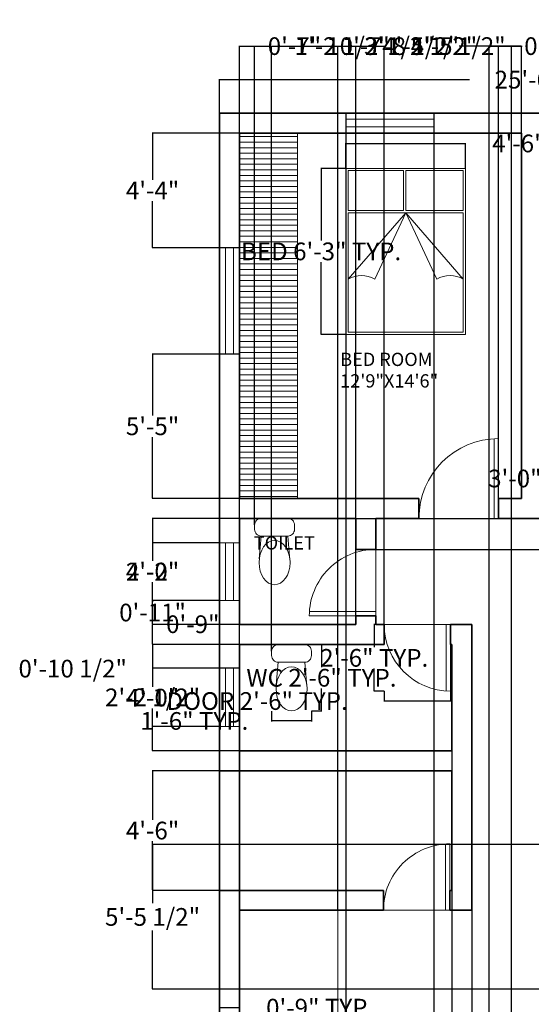
# Model space of a CAD drawing. Units: inches. Extents: x -69 to 405, y -4 to 680.
# Tile 2 of 3: x -69 to 162, y 236 to 680. Entities that reach past the tile are written whole.
import ezdxf

# ---------------------------------------------------------------- set-up
doc = ezdxf.new("R2010")
doc.units = ezdxf.units.IN
doc.header["$MEASUREMENT"] = 0
for name, color, linetype, lineweight in [('A-ANNO-DIMS', 4, 'Continuous', 18), ('A-AREA-IDEN', 4, 'Continuous', 18), ('A-FLOR-CASE', 7, 'Continuous', 18), ('A-FLOR-FIXT', 8, 'Continuous', 18), ('A-WALL', 7, 'Continuous', 35), ('Furniture', 7, 'Continuous', 15)]:
    doc.layers.add(name, color=color, linetype=linetype, lineweight=lineweight)
for name, color, linetype, lineweight, true_color in [('A-DOOR', 2, 'Continuous', 18, 0xf1eb1f), ('A-FLOR-CASE-PATT', 30, 'Continuous', 13, 0xf26722), ('A-GLAZ', 85, 'Continuous', 18, 0x58ba48)]:
    doc.layers.add(name, color=color, linetype=linetype, lineweight=lineweight, true_color=true_color)
doc.styles.get("Standard").update_dxf_attribs({"font": 'italic8.shx'})
doc.dimstyles.get("Standard").update_dxf_attribs({"dimtxt": 8, "dimasz": 0.18, "dimexe": 0.18, "dimexo": 0.0625, "dimgap": 0.09, "dimtad": 0, "dimtih": 1, "dimtoh": 1, "dimdec": 4, "dimzin": 0, "dimdsep": 46, "dimlunit": 3, "dimtxsty": 'Standard', "dimcen": 0.09, "dimadec": 0, "dimazin": 0, "dimtfac": 1, "dimtdec": 4, "dimtofl": 0, "dimtmove": 0, "dimatfit": 3, "dimfxl": 1, "dimtolj": 1, "dimtzin": 0, "dimarcsym": 0})

# ---------------------------------------------------------------- blocks, each defined once
blk = doc.blocks.new('*D4')
at = {"layer": 'A-ANNO-DIMS', "color": 0, "lineweight": -2, "transparency": 16777216}
for p, q in [((21.01, 638.35), (21.01, 653.57)), ((21.19, 653.39), (133.92, 653.39)), ((326.83, 653.39), (214.1, 653.39)), ((327.01, 638.35), (327.01, 653.57))]:
    blk.add_line(p, q, dxfattribs=at)
at = {"layer": 'A-ANNO-DIMS', "color": 0, "transparency": 16777216}
for points in [[(21.19, 653.42), (21.19, 653.36), (21.01, 653.39)], [(326.83, 653.42), (326.83, 653.36), (327.01, 653.39)]]:
    blk.add_solid(points, dxfattribs=at)
at = {"layer": 'Defpoints', "color": 0, "transparency": 16777216}
for p in [(327.01, 653.39), (21.01, 638.28), (327.01, 638.28)]:
    blk.add_point(p, dxfattribs=at)
at = {"layer": 'A-ANNO-DIMS', "color": 0, "transparency": 16777216, "insert": (174.01, 653.39), "char_height": 8, "attachment_point": 5}
blk.add_mtext('\\A1;25\'-6.0000"', dxfattribs=at)
blk = doc.blocks.new('BED-DOUBLE')
for p, q in [((26.03, 55.92), (26.03, 74)), ((27.03, 55.92), (27.03, 74)), ((1, 55.92), (26.03, 55.92)), ((1, 54.92), (53, 54.92)), ((27, 54.92), (1, 25)), ((13, 25), (27, 54.92)), ((27, 54.92), (53, 25)), ((41, 25), (27, 54.92)), ((27.03, 55.92), (53, 55.92))]:
    blk.add_line(p, q)
blk.add_lwpolyline([(0, 75), (54, 75), (54, 0), (0, 0)], close=True)
for points in [[(1, 55.92), (1, 74), (26.03, 74)], [(27.03, 74), (53, 74), (53, 55.92)], [(53, 54.92), (53, 1), (1, 1), (1, 54.92)]]:
    blk.add_lwpolyline(points)
for centre in [(7, 14.51), (47, 14.51)]:
    blk.add_arc(centre, 12.09, 60.2403, 119.7597)
blk = doc.blocks.new('WIN-48IN')
for p, q in [((0, 48), (0, 0)), ((9, 48), (0, 48)), ((2.75, 48), (2.75, 0)), ((6.25, 48), (6.25, 0)), ((9, 0), (9, 48)), ((0, 0), (9, 0))]:
    blk.add_line(p, q)
blk = doc.blocks.new('DOOR-SWING-30IN')
for p, q in [((30, 0), (0, 0)), ((0, 0), (0, -30)), ((2, 0), (2, -29.93))]:
    blk.add_line(p, q)
blk.add_arc((0, 0), 30, 270, 0)
blk = doc.blocks.new('WC-TANK')
for p, q in [((-6, 8), (-6.96, 18.89)), ((6, 8), (6.89, 18.25))]:
    blk.add_line(p, q)
blk.add_lwpolyline([(-6, 0, -0.414214), (-9, 3), (-9, 5, -0.414214), (-6, 8), (6, 8, -0.414214), (9, 5), (9, 3, -0.414214), (6, 0)], format="xyb")
blk.add_ellipse((0, 20), major_axis=(0, 10), ratio=0.7)
blk = doc.blocks.new('DOOR-SWING-36IN')
for p, q in [((0, 0), (0, 36)), ((2, 0), (2, 35.94)), ((36, 0), (0, 0))]:
    blk.add_line(p, q)
blk.add_arc((0, 0), 36, 0, 90)
blk = doc.blocks.new('*D12')
at = {"layer": 'A-ANNO-DIMS', "color": 0, "lineweight": -2, "transparency": 16777216}
for p, q in [((78.09, 613.33), (66.72, 613.33)), ((66.9, 613.15), (66.9, 580.69)), ((66.9, 538.51), (66.9, 570.98)), ((78.09, 538.33), (66.72, 538.33))]:
    blk.add_line(p, q, dxfattribs=at)
at = {"layer": 'A-ANNO-DIMS', "color": 0, "transparency": 16777216}
for points in [[(66.87, 613.15), (66.93, 613.15), (66.9, 613.33)], [(66.87, 538.51), (66.93, 538.51), (66.9, 538.33)]]:
    blk.add_solid(points, dxfattribs=at)
at = {"layer": 'Defpoints', "color": 0, "transparency": 16777216}
for p in [(66.9, 613.33), (78.15, 613.33), (78.15, 538.33)]:
    blk.add_point(p, dxfattribs=at)
at = {"layer": 'A-ANNO-DIMS', "color": 0, "transparency": 16777216, "insert": (66.9, 575.83), "char_height": 8, "attachment_point": 5}
blk.add_mtext('\\A1;BED 6\'-3" TYP.', dxfattribs=at)
blk = doc.blocks.new('*D13')
at = {"layer": 'A-ANNO-DIMS', "color": 0, "lineweight": -2, "transparency": 16777216}
for p, q in [((78.15, 613.4), (78.15, 624.76)), ((78.33, 624.58), (131.97, 624.58)), ((132.15, 613.4), (132.15, 624.76)), ((132.15, 624.58), (132.33, 624.58))]:
    blk.add_line(p, q, dxfattribs=at)
at = {"layer": 'A-ANNO-DIMS', "color": 0, "transparency": 16777216}
for points in [[(78.33, 624.61), (78.33, 624.55), (78.15, 624.58)], [(131.97, 624.61), (131.97, 624.55), (132.15, 624.58)]]:
    blk.add_solid(points, dxfattribs=at)
at = {"layer": 'Defpoints', "color": 0, "transparency": 16777216}
for p in [(132.15, 624.58), (78.15, 613.33), (132.15, 613.33)]:
    blk.add_point(p, dxfattribs=at)
at = {"layer": 'A-ANNO-DIMS', "color": 0, "transparency": 16777216, "insert": (168.61, 624.58), "char_height": 8, "attachment_point": 5}
blk.add_mtext('\\A1;4\'-6" TYP.', dxfattribs=at)
blk = doc.blocks.new('*D14')
at = {"layer": 'A-ANNO-DIMS', "color": 0, "lineweight": -2, "transparency": 16777216}
for p, q in [((62.61, 398.28), (67.23, 398.28)), ((67.05, 398.1), (67.05, 388.14)), ((67.05, 368.46), (67.05, 378.43)), ((62.61, 368.28), (67.23, 368.28))]:
    blk.add_line(p, q, dxfattribs=at)
at = {"layer": 'A-ANNO-DIMS', "color": 0, "transparency": 16777216}
for points in [[(67.02, 398.1), (67.08, 398.1), (67.05, 398.28)], [(67.02, 368.46), (67.08, 368.46), (67.05, 368.28)]]:
    blk.add_solid(points, dxfattribs=at)
at = {"layer": 'Defpoints', "color": 0, "transparency": 16777216}
for p in [(62.55, 398.28), (62.55, 368.28), (67.05, 368.28)]:
    blk.add_point(p, dxfattribs=at)
at = {"layer": 'A-ANNO-DIMS', "color": 0, "transparency": 16777216, "insert": (67.05, 383.28), "char_height": 8, "attachment_point": 5}
blk.add_mtext('\\A1;WC 2\'-6" TYP.', dxfattribs=at)
blk = doc.blocks.new('*D15')
at = {"layer": 'A-ANNO-DIMS', "color": 0, "lineweight": -2, "transparency": 16777216}
for p, q in [((44.55, 368.22), (44.55, 363.6)), ((62.55, 368.22), (62.55, 363.6)), ((44.55, 363.78), (44.37, 363.78)), ((62.37, 363.78), (44.73, 363.78))]:
    blk.add_line(p, q, dxfattribs=at)
at = {"layer": 'A-ANNO-DIMS', "color": 0, "transparency": 16777216}
for points in [[(44.73, 363.81), (44.73, 363.75), (44.55, 363.78)], [(62.37, 363.81), (62.37, 363.75), (62.55, 363.78)]]:
    blk.add_solid(points, dxfattribs=at)
at = {"layer": 'Defpoints', "color": 0, "transparency": 16777216}
for p in [(44.55, 368.28), (62.55, 368.28), (44.55, 363.78)]:
    blk.add_point(p, dxfattribs=at)
at = {"layer": 'A-ANNO-DIMS', "color": 0, "transparency": 16777216, "insert": (9.61, 363.78), "char_height": 8, "attachment_point": 5}
blk.add_mtext('\\A1;1\'-6" TYP.', dxfattribs=at)
blk = doc.blocks.new('*D17')
at = {"layer": 'A-ANNO-DIMS', "color": 0, "lineweight": -2, "transparency": 16777216}
for p, q in [((21.01, 227.18), (21.01, 234.5)), ((21.19, 234.32), (29.83, 234.32)), ((30.01, 227.18), (30.01, 234.5)), ((30.01, 234.32), (30.19, 234.32))]:
    blk.add_line(p, q, dxfattribs=at)
at = {"layer": 'A-ANNO-DIMS', "color": 0, "transparency": 16777216}
for points in [[(21.19, 234.35), (21.19, 234.29), (21.01, 234.32)], [(29.83, 234.35), (29.83, 234.29), (30.01, 234.32)]]:
    blk.add_solid(points, dxfattribs=at)
at = {"layer": 'Defpoints', "color": 0, "transparency": 16777216}
for p in [(30.01, 234.32), (21.01, 227.12), (30.01, 227.12)]:
    blk.add_point(p, dxfattribs=at)
at = {"layer": 'A-ANNO-DIMS', "color": 0, "transparency": 16777216, "insert": (66.47, 234.32), "char_height": 8, "attachment_point": 5}
blk.add_mtext('\\A1;0\'-9" TYP.', dxfattribs=at)
blk = doc.blocks.new('*D18')
at = {"layer": 'A-ANNO-DIMS', "color": 0, "lineweight": -2, "transparency": 16777216}
for p, q in [((95.41, 377.22), (95.41, 372.6)), ((125.41, 377.22), (125.41, 372.6)), ((95.41, 372.78), (95.23, 372.78)), ((125.23, 372.78), (95.59, 372.78))]:
    blk.add_line(p, q, dxfattribs=at)
at = {"layer": 'A-ANNO-DIMS', "color": 0, "transparency": 16777216}
for points in [[(95.59, 372.81), (95.59, 372.75), (95.41, 372.78)], [(125.23, 372.81), (125.23, 372.75), (125.41, 372.78)]]:
    blk.add_solid(points, dxfattribs=at)
at = {"layer": 'Defpoints', "color": 0, "transparency": 16777216}
for p in [(95.41, 377.28), (125.41, 377.28), (95.41, 372.78)]:
    blk.add_point(p, dxfattribs=at)
at = {"layer": 'A-ANNO-DIMS', "color": 0, "transparency": 16777216, "insert": (37.99, 372.78), "char_height": 8, "attachment_point": 5}
blk.add_mtext('\\A1;DOOR 2\'-6" TYP.', dxfattribs=at)
blk = doc.blocks.new('*D19')
at = {"layer": 'A-ANNO-DIMS', "color": 0, "lineweight": -2, "transparency": 16777216}
for p, q in [((95.34, 407.28), (90.73, 407.28)), ((90.91, 407.1), (90.91, 397.14)), ((90.91, 377.46), (90.91, 387.43)), ((95.34, 377.28), (90.73, 377.28))]:
    blk.add_line(p, q, dxfattribs=at)
at = {"layer": 'A-ANNO-DIMS', "color": 0, "transparency": 16777216}
for points in [[(90.88, 407.1), (90.94, 407.1), (90.91, 407.28)], [(90.88, 377.46), (90.94, 377.46), (90.91, 377.28)]]:
    blk.add_solid(points, dxfattribs=at)
at = {"layer": 'Defpoints', "color": 0, "transparency": 16777216}
for p in [(90.91, 407.28), (95.41, 407.28), (95.41, 377.28)]:
    blk.add_point(p, dxfattribs=at)
at = {"layer": 'A-ANNO-DIMS', "color": 0, "transparency": 16777216, "insert": (90.91, 392.28), "char_height": 8, "attachment_point": 5}
blk.add_mtext('\\A1;2\'-6" TYP.', dxfattribs=at)
blk = doc.blocks.new('*D21')
at = {"layer": 'A-ANNO-DIMS', "color": 0, "lineweight": -2, "transparency": 16777216}
for p, q in [((172.14, 491.28), (166.62, 491.28)), ((166.8, 491.1), (166.8, 478.14)), ((166.8, 455.46), (166.8, 468.43)), ((172.14, 455.28), (166.62, 455.28))]:
    blk.add_line(p, q, dxfattribs=at)
at = {"layer": 'A-ANNO-DIMS', "color": 0, "transparency": 16777216}
for points in [[(166.77, 491.1), (166.83, 491.1), (166.8, 491.28)], [(166.77, 455.46), (166.83, 455.46), (166.8, 455.28)]]:
    blk.add_solid(points, dxfattribs=at)
at = {"layer": 'Defpoints', "color": 0, "transparency": 16777216}
for p in [(166.8, 491.28), (172.2, 491.28), (172.2, 455.28)]:
    blk.add_point(p, dxfattribs=at)
at = {"layer": 'A-ANNO-DIMS', "color": 0, "transparency": 16777216, "insert": (166.8, 473.28), "char_height": 8, "attachment_point": 5}
blk.add_mtext('\\A1;3\'-0" TYP.', dxfattribs=at)
blk = doc.blocks.new('*D28')
at = {"layer": 'A-ANNO-DIMS', "color": 0, "lineweight": -2, "transparency": 16777216}
for p, q in [((142.9, 125.35), (142.9, 668.71)), ((143.08, 668.53), (152.72, 668.53)), ((152.9, 125.35), (152.9, 668.71)), ((152.9, 668.53), (153.08, 668.53))]:
    blk.add_line(p, q, dxfattribs=at)
at = {"layer": 'A-ANNO-DIMS', "color": 0, "transparency": 16777216}
for points in [[(143.08, 668.56), (143.08, 668.5), (142.9, 668.53)], [(152.72, 668.56), (152.72, 668.5), (152.9, 668.53)]]:
    blk.add_solid(points, dxfattribs=at)
at = {"layer": 'Defpoints', "color": 0, "transparency": 16777216}
for p in [(152.9, 668.53), (142.9, 125.28), (152.9, 125.28)]:
    blk.add_point(p, dxfattribs=at)
at = {"layer": 'A-ANNO-DIMS', "color": 0, "transparency": 16777216, "insert": (173.75, 668.53), "char_height": 8, "attachment_point": 5}
blk.add_mtext('\\A1;0\'-10"', dxfattribs=at)
blk = doc.blocks.new('*D33')
at = {"layer": 'A-ANNO-DIMS', "color": 0, "lineweight": -2, "transparency": 16777216}
for p, q in [((30.01, 350.22), (30.01, 7.85)), ((126.01, 350.22), (126.01, 7.85)), ((30.19, 8.03), (60.01, 8.03)), ((125.83, 8.03), (96, 8.03))]:
    blk.add_line(p, q, dxfattribs=at)
at = {"layer": 'A-ANNO-DIMS', "color": 0, "transparency": 16777216}
for points in [[(30.19, 8.06), (30.19, 8), (30.01, 8.03)], [(125.83, 8.06), (125.83, 8), (126.01, 8.03)]]:
    blk.add_solid(points, dxfattribs=at)
at = {"layer": 'Defpoints', "color": 0, "transparency": 16777216}
for p in [(30.01, 350.28), (126.01, 350.28), (126.01, 8.03)]:
    blk.add_point(p, dxfattribs=at)
at = {"layer": 'A-ANNO-DIMS', "color": 0, "transparency": 16777216, "insert": (78.01, 8.03), "char_height": 8, "attachment_point": 5}
blk.add_mtext('\\A1;8\'-0"', dxfattribs=at)
blk = doc.blocks.new('*D34')
at = {"layer": 'A-ANNO-DIMS', "color": 0, "lineweight": -2, "transparency": 16777216}
for p, q in [((29.95, 398.28), (-9.42, 398.28)), ((-9.24, 398.1), (-9.24, 379.14)), ((-9.24, 350.46), (-9.24, 369.43)), ((29.95, 350.28), (-9.42, 350.28))]:
    blk.add_line(p, q, dxfattribs=at)
at = {"layer": 'A-ANNO-DIMS', "color": 0, "transparency": 16777216}
for points in [[(-9.27, 398.1), (-9.21, 398.1), (-9.24, 398.28)], [(-9.27, 350.46), (-9.21, 350.46), (-9.24, 350.28)]]:
    blk.add_solid(points, dxfattribs=at)
at = {"layer": 'Defpoints', "color": 0, "transparency": 16777216}
for p in [(-9.24, 398.28), (30.01, 398.28), (30.01, 350.28)]:
    blk.add_point(p, dxfattribs=at)
at = {"layer": 'A-ANNO-DIMS', "color": 0, "transparency": 16777216, "insert": (-9.24, 374.28), "char_height": 8, "attachment_point": 5}
blk.add_mtext('\\A1;4\'-0"', dxfattribs=at)
blk = doc.blocks.new('*D35')
at = {"layer": 'A-ANNO-DIMS', "color": 0, "lineweight": -2, "transparency": 16777216}
for p, q in [((30.01, 407.35), (30.01, 668.71)), ((30.19, 668.53), (82.38, 668.53)), ((82.56, 407.35), (82.56, 668.71)), ((82.56, 668.53), (82.74, 668.53))]:
    blk.add_line(p, q, dxfattribs=at)
at = {"layer": 'A-ANNO-DIMS', "color": 0, "transparency": 16777216}
for points in [[(30.19, 668.56), (30.19, 668.5), (30.01, 668.53)], [(82.38, 668.56), (82.38, 668.5), (82.56, 668.53)]]:
    blk.add_solid(points, dxfattribs=at)
at = {"layer": 'Defpoints', "color": 0, "transparency": 16777216}
for p in [(82.56, 668.53), (30.01, 407.28), (82.56, 407.28)]:
    blk.add_point(p, dxfattribs=at)
at = {"layer": 'A-ANNO-DIMS', "color": 0, "transparency": 16777216, "insert": (115.98, 668.53), "char_height": 8, "attachment_point": 5}
blk.add_mtext('\\A1;4\'-4 1/2"', dxfattribs=at)
blk = doc.blocks.new('*D36')
at = {"layer": 'A-ANNO-DIMS', "color": 0, "lineweight": -2, "transparency": 16777216}
for p, q in [((29.95, 455.28), (-9.42, 455.28)), ((-9.24, 455.1), (-9.24, 436.14)), ((-9.24, 407.46), (-9.24, 426.43)), ((29.95, 407.28), (-9.42, 407.28))]:
    blk.add_line(p, q, dxfattribs=at)
at = {"layer": 'A-ANNO-DIMS', "color": 0, "transparency": 16777216}
for points in [[(-9.27, 455.1), (-9.21, 455.1), (-9.24, 455.28)], [(-9.27, 407.46), (-9.21, 407.46), (-9.24, 407.28)]]:
    blk.add_solid(points, dxfattribs=at)
at = {"layer": 'Defpoints', "color": 0, "transparency": 16777216}
for p in [(-9.24, 455.28), (30.01, 455.28), (30.01, 407.28)]:
    blk.add_point(p, dxfattribs=at)
at = {"layer": 'A-ANNO-DIMS', "color": 0, "transparency": 16777216, "insert": (-9.24, 431.28), "char_height": 8, "attachment_point": 5}
blk.add_mtext('\\A1;4\'-0"', dxfattribs=at)
blk = doc.blocks.new('*D39')
at = {"layer": 'A-ANNO-DIMS', "color": 0, "lineweight": -2, "transparency": 16777216}
for p, q in [((20.95, 341.28), (-9.42, 341.28)), ((-9.24, 341.1), (-9.24, 319.14)), ((-9.24, 287.46), (-9.24, 309.43)), ((20.95, 287.28), (-9.42, 287.28))]:
    blk.add_line(p, q, dxfattribs=at)
at = {"layer": 'A-ANNO-DIMS', "color": 0, "transparency": 16777216}
for points in [[(-9.27, 341.1), (-9.21, 341.1), (-9.24, 341.28)], [(-9.27, 287.46), (-9.21, 287.46), (-9.24, 287.28)]]:
    blk.add_solid(points, dxfattribs=at)
at = {"layer": 'Defpoints', "color": 0, "transparency": 16777216}
for p in [(21.01, 341.28), (-9.24, 287.28), (21.01, 287.28)]:
    blk.add_point(p, dxfattribs=at)
at = {"layer": 'A-ANNO-DIMS', "color": 0, "transparency": 16777216, "insert": (-9.24, 314.28), "char_height": 8, "attachment_point": 5}
blk.add_mtext('\\A1;4\'-6"', dxfattribs=at)
blk = doc.blocks.new('*D40')
at = {"layer": 'A-ANNO-DIMS', "color": 0, "lineweight": -2, "transparency": 16777216}
for p, q in [((135.01, 407.22), (135.01, 7.85)), ((183.01, 407.22), (183.01, 7.85)), ((135.19, 8.03), (141.01, 8.03)), ((182.83, 8.03), (177, 8.03))]:
    blk.add_line(p, q, dxfattribs=at)
at = {"layer": 'A-ANNO-DIMS', "color": 0, "transparency": 16777216}
for points in [[(135.19, 8.06), (135.19, 8), (135.01, 8.03)], [(182.83, 8.06), (182.83, 8), (183.01, 8.03)]]:
    blk.add_solid(points, dxfattribs=at)
at = {"layer": 'Defpoints', "color": 0, "transparency": 16777216}
for p in [(135.01, 407.28), (183.01, 407.28), (183.01, 8.03)]:
    blk.add_point(p, dxfattribs=at)
at = {"layer": 'A-ANNO-DIMS', "color": 0, "transparency": 16777216, "insert": (159.01, 8.03), "char_height": 8, "attachment_point": 5}
blk.add_mtext('\\A1;4\'-0"', dxfattribs=at)
blk = doc.blocks.new('*D41')
at = {"layer": 'A-ANNO-DIMS', "color": 0, "lineweight": -2, "transparency": 16777216}
for p, q in [((30.01, 629.35), (30.01, 668.71)), ((30.19, 668.53), (58.24, 668.53)), ((157.33, 668.53), (129.28, 668.53)), ((157.51, 629.35), (157.51, 668.71))]:
    blk.add_line(p, q, dxfattribs=at)
at = {"layer": 'A-ANNO-DIMS', "color": 0, "transparency": 16777216}
for points in [[(30.19, 668.56), (30.19, 668.5), (30.01, 668.53)], [(157.33, 668.56), (157.33, 668.5), (157.51, 668.53)]]:
    blk.add_solid(points, dxfattribs=at)
at = {"layer": 'Defpoints', "color": 0, "transparency": 16777216}
for p in [(157.51, 668.53), (30.01, 629.28), (157.51, 629.28)]:
    blk.add_point(p, dxfattribs=at)
at = {"layer": 'A-ANNO-DIMS', "color": 0, "transparency": 16777216, "insert": (93.76, 668.53), "char_height": 8, "attachment_point": 5}
blk.add_mtext('\\A1;10\'-7 1/2"', dxfattribs=at)
blk = doc.blocks.new('*D43')
at = {"layer": 'A-ANNO-DIMS', "color": 0, "lineweight": -2, "transparency": 16777216}
for p, q in [((29.95, 529.44), (-9.42, 529.44)), ((-9.24, 529.26), (-9.24, 501.71)), ((-9.24, 464.46), (-9.24, 492.01)), ((29.95, 464.28), (-9.42, 464.28))]:
    blk.add_line(p, q, dxfattribs=at)
at = {"layer": 'A-ANNO-DIMS', "color": 0, "transparency": 16777216}
for points in [[(-9.27, 529.26), (-9.21, 529.26), (-9.24, 529.44)], [(-9.27, 464.46), (-9.21, 464.46), (-9.24, 464.28)]]:
    blk.add_solid(points, dxfattribs=at)
at = {"layer": 'Defpoints', "color": 0, "transparency": 16777216}
for p in [(-9.24, 529.44), (30.01, 529.44), (30.01, 464.28)]:
    blk.add_point(p, dxfattribs=at)
at = {"layer": 'A-ANNO-DIMS', "color": 0, "transparency": 16777216, "insert": (-9.24, 496.86), "char_height": 8, "attachment_point": 5}
blk.add_mtext('\\A1;5\'-5"', dxfattribs=at)
blk = doc.blocks.new('*D44')
at = {"layer": 'A-ANNO-DIMS', "color": 0, "lineweight": -2, "transparency": 16777216}
for p, q in [((21.01, 638.22), (21.01, 7.85)), ((78.06, 638.22), (78.06, 7.85)), ((21.19, 8.03), (31.54, 8.03)), ((77.88, 8.03), (67.53, 8.03))]:
    blk.add_line(p, q, dxfattribs=at)
at = {"layer": 'A-ANNO-DIMS', "color": 0, "transparency": 16777216}
for points in [[(21.19, 8.06), (21.19, 8), (21.01, 8.03)], [(77.88, 8.06), (77.88, 8), (78.06, 8.03)]]:
    blk.add_solid(points, dxfattribs=at)
at = {"layer": 'Defpoints', "color": 0, "transparency": 16777216}
for p in [(21.01, 638.28), (78.06, 638.28), (78.06, 8.03)]:
    blk.add_point(p, dxfattribs=at)
at = {"layer": 'A-ANNO-DIMS', "color": 0, "transparency": 16777216, "insert": (49.53, 8.03), "char_height": 8, "attachment_point": 5}
blk.add_mtext('\\A1;4\'-9"', dxfattribs=at)
blk = doc.blocks.new('*D45')
at = {"layer": 'A-ANNO-DIMS', "color": 0, "lineweight": -2, "transparency": 16777216}
for p, q in [((78.06, 638.22), (78.06, 7.85)), ((117.87, 638.22), (117.87, 7.85)), ((78.24, 8.03), (79.97, 8.03)), ((117.69, 8.03), (115.96, 8.03))]:
    blk.add_line(p, q, dxfattribs=at)
at = {"layer": 'A-ANNO-DIMS', "color": 0, "transparency": 16777216}
for points in [[(78.24, 8.06), (78.24, 8), (78.06, 8.03)], [(117.69, 8.06), (117.69, 8), (117.87, 8.03)]]:
    blk.add_solid(points, dxfattribs=at)
at = {"layer": 'Defpoints', "color": 0, "transparency": 16777216}
for p in [(78.06, 638.28), (117.87, 638.28), (117.87, 8.03)]:
    blk.add_point(p, dxfattribs=at)
at = {"layer": 'A-ANNO-DIMS', "color": 0, "transparency": 16777216, "insert": (97.96, 8.03), "char_height": 8, "attachment_point": 5}
blk.add_mtext('\\A1;3\'-4"', dxfattribs=at)
blk = doc.blocks.new('*D48')
at = {"layer": 'A-ANNO-DIMS', "color": 0, "lineweight": -2, "transparency": 16777216}
for p, q in [((29.95, 629.28), (-9.42, 629.28)), ((-9.24, 629.1), (-9.24, 608.21)), ((-9.24, 577.62), (-9.24, 598.51)), ((29.95, 577.44), (-9.42, 577.44))]:
    blk.add_line(p, q, dxfattribs=at)
at = {"layer": 'A-ANNO-DIMS', "color": 0, "transparency": 16777216}
for points in [[(-9.27, 629.1), (-9.21, 629.1), (-9.24, 629.28)], [(-9.27, 577.62), (-9.21, 577.62), (-9.24, 577.44)]]:
    blk.add_solid(points, dxfattribs=at)
at = {"layer": 'Defpoints', "color": 0, "transparency": 16777216}
for p in [(30.01, 629.28), (-9.24, 577.44), (30.01, 577.44)]:
    blk.add_point(p, dxfattribs=at)
at = {"layer": 'A-ANNO-DIMS', "color": 0, "transparency": 16777216, "insert": (-9.24, 603.36), "char_height": 8, "attachment_point": 5}
blk.add_mtext('\\A1;4\'-4"', dxfattribs=at)
blk = doc.blocks.new('*D52')
at = {"layer": 'A-ANNO-DIMS', "color": 0, "lineweight": -2, "transparency": 16777216}
for p, q in [((147.12, 464.35), (147.12, 668.71)), ((147.3, 668.53), (157.33, 668.53)), ((157.51, 464.35), (157.51, 668.71)), ((157.51, 668.53), (157.69, 668.53))]:
    blk.add_line(p, q, dxfattribs=at)
at = {"layer": 'A-ANNO-DIMS', "color": 0, "transparency": 16777216}
for points in [[(147.3, 668.56), (147.3, 668.5), (147.12, 668.53)], [(157.33, 668.56), (157.33, 668.5), (157.51, 668.53)]]:
    blk.add_solid(points, dxfattribs=at)
at = {"layer": 'Defpoints', "color": 0, "transparency": 16777216}
for p in [(157.51, 668.53), (147.12, 464.28), (157.51, 464.28)]:
    blk.add_point(p, dxfattribs=at)
at = {"layer": 'A-ANNO-DIMS', "color": 0, "transparency": 16777216, "insert": (193.59, 668.53), "char_height": 8, "attachment_point": 5}
blk.add_mtext('\\A1;0\'-10 1/2"', dxfattribs=at)
blk = doc.blocks.new('*D54')
at = {"layer": 'A-ANNO-DIMS', "color": 0, "lineweight": -2, "transparency": 16777216}
for p, q in [((20.95, 444.18), (-9.42, 444.18)), ((-9.24, 444), (-9.24, 436.04)), ((-9.24, 418.38), (-9.24, 426.34)), ((20.95, 418.2), (-9.42, 418.2))]:
    blk.add_line(p, q, dxfattribs=at)
at = {"layer": 'A-ANNO-DIMS', "color": 0, "transparency": 16777216}
for points in [[(-9.27, 444), (-9.21, 444), (-9.24, 444.18)], [(-9.27, 418.38), (-9.21, 418.38), (-9.24, 418.2)]]:
    blk.add_solid(points, dxfattribs=at)
at = {"layer": 'Defpoints', "color": 0, "transparency": 16777216}
for p in [(-9.24, 444.18), (21.01, 444.18), (21.01, 418.2)]:
    blk.add_point(p, dxfattribs=at)
at = {"layer": 'A-ANNO-DIMS', "color": 0, "transparency": 16777216, "insert": (-9.24, 431.19), "char_height": 8, "attachment_point": 5}
blk.add_mtext('\\A1;2\'-2"', dxfattribs=at)
blk = doc.blocks.new('*D55')
at = {"layer": 'A-ANNO-DIMS', "color": 0, "lineweight": -2, "transparency": 16777216}
for p, q in [((20.95, 387.59), (-9.42, 387.59)), ((-9.24, 387.41), (-9.24, 380.61)), ((-9.24, 361.45), (-9.24, 368.24)), ((20.95, 361.27), (-9.42, 361.27))]:
    blk.add_line(p, q, dxfattribs=at)
at = {"layer": 'A-ANNO-DIMS', "color": 0, "transparency": 16777216}
for points in [[(-9.27, 387.41), (-9.21, 387.41), (-9.24, 387.59)], [(-9.27, 361.45), (-9.21, 361.45), (-9.24, 361.27)]]:
    blk.add_solid(points, dxfattribs=at)
at = {"layer": 'Defpoints', "color": 0, "transparency": 16777216}
for p in [(-9.24, 387.59), (21.01, 387.59), (21.01, 361.27)]:
    blk.add_point(p, dxfattribs=at)
at = {"layer": 'A-ANNO-DIMS', "color": 0, "transparency": 16777216, "insert": (-9.24, 374.43), "char_height": 8, "attachment_point": 5}
blk.add_mtext('\\A1;2\'-2 1/2"', dxfattribs=at)
blk = doc.blocks.new('*D57')
at = {"layer": 'A-ANNO-DIMS', "color": 0, "lineweight": -2, "transparency": 16777216}
for p, q in [((20.95, 418.2), (-9.42, 418.2)), ((-9.24, 418.02), (-9.24, 417.6)), ((29.95, 407.28), (-9.42, 407.28)), ((-9.24, 407.46), (-9.24, 407.89))]:
    blk.add_line(p, q, dxfattribs=at)
at = {"layer": 'A-ANNO-DIMS', "color": 0, "transparency": 16777216}
for points in [[(-9.27, 418.02), (-9.21, 418.02), (-9.24, 418.2)], [(-9.27, 407.46), (-9.21, 407.46), (-9.24, 407.28)]]:
    blk.add_solid(points, dxfattribs=at)
at = {"layer": 'Defpoints', "color": 0, "transparency": 16777216}
for p in [(-9.24, 418.2), (21.01, 418.2), (30.01, 407.28)]:
    blk.add_point(p, dxfattribs=at)
at = {"layer": 'A-ANNO-DIMS', "color": 0, "transparency": 16777216, "insert": (-9.24, 412.74), "char_height": 8, "attachment_point": 5}
blk.add_mtext('\\A1;0\'-11"', dxfattribs=at)
blk = doc.blocks.new('*D58')
at = {"layer": 'A-ANNO-DIMS', "color": 0, "lineweight": -2, "transparency": 16777216}
for p, q in [((29.95, 398.28), (-9.42, 398.28)), ((-9.24, 398.1), (-9.24, 387.77)), ((29.95, 387.59), (-9.42, 387.59)), ((-9.24, 387.41), (-9.42, 387.41)), ((-9.24, 387.59), (-9.24, 387.41))]:
    blk.add_line(p, q, dxfattribs=at)
at = {"layer": 'A-ANNO-DIMS', "color": 0, "transparency": 16777216}
for points in [[(-9.27, 398.1), (-9.21, 398.1), (-9.24, 398.28)], [(-9.27, 387.77), (-9.21, 387.77), (-9.24, 387.59)]]:
    blk.add_solid(points, dxfattribs=at)
at = {"layer": 'Defpoints', "color": 0, "transparency": 16777216}
for p in [(30.01, 398.28), (-9.24, 387.59), (30.01, 387.59)]:
    blk.add_point(p, dxfattribs=at)
at = {"layer": 'A-ANNO-DIMS', "color": 0, "transparency": 16777216, "insert": (-45.32, 387.41), "char_height": 8, "attachment_point": 5}
blk.add_mtext('\\A1;0\'-10 1/2"', dxfattribs=at)
blk = doc.blocks.new('*D59')
at = {"layer": 'A-ANNO-DIMS', "color": 0, "lineweight": -2, "transparency": 16777216}
for p, q in [((30.01, 398.35), (30.01, 668.71)), ((30.19, 668.53), (44.37, 668.53)), ((44.55, 395.35), (44.55, 668.71)), ((44.55, 668.53), (44.73, 668.53))]:
    blk.add_line(p, q, dxfattribs=at)
at = {"layer": 'A-ANNO-DIMS', "color": 0, "transparency": 16777216}
for points in [[(30.19, 668.56), (30.19, 668.5), (30.01, 668.53)], [(44.37, 668.56), (44.37, 668.5), (44.55, 668.53)]]:
    blk.add_solid(points, dxfattribs=at)
at = {"layer": 'Defpoints', "color": 0, "transparency": 16777216}
for p in [(44.55, 668.53), (30.01, 398.28), (44.55, 395.28)]:
    blk.add_point(p, dxfattribs=at)
at = {"layer": 'A-ANNO-DIMS', "color": 0, "transparency": 16777216, "insert": (76.43, 668.53), "char_height": 8, "attachment_point": 5}
blk.add_mtext('\\A1;1\'-2 1/2"', dxfattribs=at)
blk = doc.blocks.new('*D60')
at = {"layer": 'A-ANNO-DIMS', "color": 0, "lineweight": -2, "transparency": 16777216}
for p, q in [((30.01, 455.35), (30.01, 668.71)), ((30.19, 668.53), (36.69, 668.53)), ((36.87, 452.35), (36.87, 668.71)), ((36.87, 668.53), (37.05, 668.53))]:
    blk.add_line(p, q, dxfattribs=at)
at = {"layer": 'A-ANNO-DIMS', "color": 0, "transparency": 16777216}
for points in [[(30.19, 668.56), (30.19, 668.5), (30.01, 668.53)], [(36.69, 668.56), (36.69, 668.5), (36.87, 668.53)]]:
    blk.add_solid(points, dxfattribs=at)
at = {"layer": 'Defpoints', "color": 0, "transparency": 16777216}
for p in [(36.87, 668.53), (30.01, 455.28), (36.87, 452.28)]:
    blk.add_point(p, dxfattribs=at)
at = {"layer": 'A-ANNO-DIMS', "color": 0, "transparency": 16777216, "insert": (54.85, 668.53), "char_height": 8, "attachment_point": 5}
blk.add_mtext('\\A1;0\'-7"', dxfattribs=at)
blk = doc.blocks.new('*D61')
at = {"layer": 'A-ANNO-DIMS', "color": 0, "lineweight": -2, "transparency": 16777216}
for p, q in [((82.63, 455.28), (357.44, 455.28)), ((357.26, 455.1), (357.26, 453.13)), ((82.63, 441.28), (357.44, 441.28)), ((357.26, 441.46), (357.26, 443.43))]:
    blk.add_line(p, q, dxfattribs=at)
at = {"layer": 'A-ANNO-DIMS', "color": 0, "transparency": 16777216}
for points in [[(357.23, 455.1), (357.29, 455.1), (357.26, 455.28)], [(357.23, 441.46), (357.29, 441.46), (357.26, 441.28)]]:
    blk.add_solid(points, dxfattribs=at)
at = {"layer": 'Defpoints', "color": 0, "transparency": 16777216}
for p in [(82.56, 455.28), (82.56, 441.28), (357.26, 441.28)]:
    blk.add_point(p, dxfattribs=at)
at = {"layer": 'A-ANNO-DIMS', "color": 0, "transparency": 16777216, "insert": (357.26, 448.28), "char_height": 8, "attachment_point": 5}
blk.add_mtext('\\A1;1\'-2"', dxfattribs=at)
blk = doc.blocks.new('*D62')
at = {"layer": 'A-ANNO-DIMS', "color": 0, "lineweight": -2, "transparency": 16777216}
for p, q in [((30.01, 398.35), (30.01, 668.71)), ((30.19, 668.53), (95.23, 668.53)), ((95.41, 398.35), (95.41, 668.71)), ((95.41, 668.53), (95.59, 668.53))]:
    blk.add_line(p, q, dxfattribs=at)
at = {"layer": 'A-ANNO-DIMS', "color": 0, "transparency": 16777216}
for points in [[(30.19, 668.56), (30.19, 668.5), (30.01, 668.53)], [(95.23, 668.56), (95.23, 668.5), (95.41, 668.53)]]:
    blk.add_solid(points, dxfattribs=at)
at = {"layer": 'Defpoints', "color": 0, "transparency": 16777216}
for p in [(95.41, 668.53), (30.01, 398.28), (95.41, 398.28)]:
    blk.add_point(p, dxfattribs=at)
at = {"layer": 'A-ANNO-DIMS', "color": 0, "transparency": 16777216, "insert": (128.82, 668.53), "char_height": 8, "attachment_point": 5}
blk.add_mtext('\\A1;5\'-5 1/2"', dxfattribs=at)
blk = doc.blocks.new('*D63')
at = {"layer": 'A-ANNO-DIMS', "color": 0, "lineweight": -2, "transparency": 16777216}
for p, q in [((30.01, 278.35), (30.01, 668.71)), ((30.19, 668.53), (74.21, 668.53)), ((74.39, 278.35), (74.39, 668.71)), ((74.39, 668.53), (74.57, 668.53))]:
    blk.add_line(p, q, dxfattribs=at)
at = {"layer": 'A-ANNO-DIMS', "color": 0, "transparency": 16777216}
for points in [[(30.19, 668.56), (30.19, 668.5), (30.01, 668.53)], [(74.21, 668.56), (74.21, 668.5), (74.39, 668.53)]]:
    blk.add_solid(points, dxfattribs=at)
at = {"layer": 'Defpoints', "color": 0, "transparency": 16777216}
for p in [(74.39, 668.53), (30.01, 278.28), (74.39, 278.28)]:
    blk.add_point(p, dxfattribs=at)
at = {"layer": 'A-ANNO-DIMS', "color": 0, "transparency": 16777216, "insert": (107.81, 668.53), "char_height": 8, "attachment_point": 5}
blk.add_mtext('\\A1;3\'-8 1/2"', dxfattribs=at)
blk = doc.blocks.new('*D66')
at = {"layer": 'A-ANNO-DIMS', "color": 0, "lineweight": -2, "transparency": 16777216}
for p, q in [((182.95, 307.92), (-9.42, 307.92)), ((-9.24, 307.74), (-9.24, 281.48)), ((-9.24, 242.85), (-9.24, 269.11)), ((182.95, 242.67), (-9.42, 242.67))]:
    blk.add_line(p, q, dxfattribs=at)
at = {"layer": 'A-ANNO-DIMS', "color": 0, "transparency": 16777216}
for points in [[(-9.27, 307.74), (-9.21, 307.74), (-9.24, 307.92)], [(-9.27, 242.85), (-9.21, 242.85), (-9.24, 242.67)]]:
    blk.add_solid(points, dxfattribs=at)
at = {"layer": 'Defpoints', "color": 0, "transparency": 16777216}
for p in [(-9.24, 307.92), (183.01, 307.92), (183.01, 242.67)]:
    blk.add_point(p, dxfattribs=at)
at = {"layer": 'A-ANNO-DIMS', "color": 0, "transparency": 16777216, "insert": (-9.24, 275.29), "char_height": 8, "attachment_point": 5}
blk.add_mtext('\\A1;5\'-5 1/2"', dxfattribs=at)
blk = doc.blocks.new('*D67')
at = {"layer": 'A-ANNO-DIMS', "color": 0, "lineweight": -2, "transparency": 16777216}
for p, q in [((29.95, 407.28), (-9.42, 407.28)), ((-9.24, 407.28), (-9.24, 407.46)), ((-9.24, 407.46), (-9.06, 407.46)), ((-9.24, 398.46), (-9.24, 407.1)), ((29.95, 398.28), (-9.42, 398.28))]:
    blk.add_line(p, q, dxfattribs=at)
at = {"layer": 'A-ANNO-DIMS', "color": 0, "transparency": 16777216}
for points in [[(-9.27, 407.1), (-9.21, 407.1), (-9.24, 407.28)], [(-9.27, 398.46), (-9.21, 398.46), (-9.24, 398.28)]]:
    blk.add_solid(points, dxfattribs=at)
at = {"layer": 'Defpoints', "color": 0, "transparency": 16777216}
for p in [(-9.24, 407.28), (30.01, 407.28), (30.01, 398.28)]:
    blk.add_point(p, dxfattribs=at)
at = {"layer": 'A-ANNO-DIMS', "color": 0, "transparency": 16777216, "insert": (8.93, 407.46), "char_height": 8, "attachment_point": 5}
blk.add_mtext('\\A1;0\'-9"', dxfattribs=at)

msp = doc.modelspace()

# ---------------------------------------------------------------- hatches: boundary and pattern name
at = {"layer": 'A-FLOR-CASE-PATT'}
h = msp.add_hatch(dxfattribs=at)
h.set_pattern_fill('LINE', color=256, scale=20)
h.set_pattern_definition([(0, (-346.6938, -34.8461), (0, 2.5), [])])
h.paths.add_polyline_path([(56.30318, 629.28441), (30.00851, 629.28441), (30.00851, 464.28441), (56.30318, 464.28441)])
h.paths.add_polyline_path([(318.00851, 629.28441), (293.21188, 629.28441), (293.21188, 464.28441), (318.00851, 464.28441)])

# ---------------------------------------------------------------- linework, layer by layer
at = {"layer": 'A-FLOR-CASE'}
for p, q in [((56.30318, 464.28441), (56.30318, 629.28441)), ((74.39466, 278.28441), (74.39466, 166.22496))]:
    msp.add_line(p, q, dxfattribs=at)
at = {"layer": 'A-GLAZ'}
for p, q in [((78.0556, 638.28441), (78.0556, 629.28441)), ((117.8737, 638.28441), (78.0556, 638.28441)), ((117.8737, 629.28441), (117.8737, 638.28441)), ((78.0556, 635.53441), (117.8737, 635.53441)), ((78.0556, 632.03441), (117.8737, 632.03441)), ((78.0556, 629.28441), (117.8737, 629.28441)), ((30.00851, 444.18093), (21.00851, 444.18093)), ((21.00851, 444.18093), (21.00851, 418.20227)), ((23.75851, 444.18093), (23.75851, 418.20227)), ((27.25851, 444.18093), (27.25851, 418.20227)), ((30.00851, 418.20227), (30.00851, 444.18093)), ((21.00851, 418.20227), (30.00851, 418.20227)), ((30.00851, 387.58967), (21.00851, 387.58967)), ((21.00851, 387.58967), (21.00851, 361.26799)), ((23.75851, 387.58967), (23.75851, 361.26799)), ((27.25851, 387.58967), (27.25851, 361.26799)), ((30.00851, 361.26799), (30.00851, 387.58967)), ((21.00851, 361.26799), (30.00851, 361.26799))]:
    msp.add_line(p, q, dxfattribs=at)
at = {"layer": 'A-WALL'}
for p, q in [((30.00851, 629.28441), (30.00851, 464.28441)), ((157.50851, 629.28441), (30.00851, 629.28441)), ((157.50851, 464.28441), (157.50851, 629.28441)), ((111.11856, 464.28441), (30.00851, 464.28441)), ((111.11856, 464.28441), (111.11856, 455.28441)), ((157.50851, 464.28441), (147.11856, 464.28441)), ((147.11856, 464.28441), (147.11856, 455.28441)), ((30.00851, 455.28441), (30.00851, 407.28441)), ((82.56355, 455.28441), (30.00851, 455.28441)), ((82.56355, 455.28441), (82.56355, 441.28014)), ((91.56355, 455.28441), (91.56355, 441.28014)), ((111.11856, 455.28441), (91.56355, 455.28441)), ((172.20116, 455.28441), (147.11856, 455.28441)), ((91.56355, 441.28014), (82.56355, 441.28014)), ((91.56355, 411.28014), (82.56355, 411.28014)), ((82.56355, 411.28014), (82.56355, 407.28441)), ((91.56355, 411.28014), (91.56355, 407.28441)), ((82.56355, 407.28441), (30.00851, 407.28441)), ((95.40533, 407.28441), (91.56355, 407.28441)), ((95.40533, 398.28441), (95.40533, 407.28441)), ((125.40533, 398.28441), (125.40533, 407.28441)), ((135.00851, 407.28441), (125.40533, 407.28441)), ((135.00851, 407.28441), (135.00851, 278.28441)), ((30.00851, 398.28441), (30.00851, 350.28441)), ((95.40533, 398.28441), (30.00851, 398.28441)), ((126.00851, 398.28441), (125.40533, 398.28441)), ((126.00851, 398.28441), (126.00851, 350.28441)), ((126.00851, 350.28441), (30.00851, 350.28441)), ((126.00851, 341.28441), (21.00851, 341.28441)), ((126.00851, 341.28441), (126.00851, 287.28441)), ((21.00851, 287.28441), (95.06807, 287.28441)), ((95.06807, 278.28441), (95.06807, 287.28441)), ((125.06807, 278.28441), (125.06807, 287.28441)), ((125.06807, 287.28441), (126.00851, 287.28441)), ((30.00851, 278.28441), (95.06807, 278.28441)), ((30.00851, 278.28441), (30.00851, 134.28441)), ((125.06807, 278.28441), (135.00851, 278.28441))]:
    msp.add_line(p, q, dxfattribs=at)
msp.add_lwpolyline([(21.00851, 38.28441), (327.00851, 38.28441), (327.00851, 638.28441), (21.00851, 638.28441)], close=True, dxfattribs=at)

# ---------------------------------------------------------------- block references
at = {"layer": 'A-DOOR', "extrusion": (0, 0, -1), "zscale": -1}
for name, p in [('DOOR-SWING-36IN', (-147.11856, 455.28441)), ('DOOR-SWING-30IN', (-125.40533, 407.28441))]:
    msp.add_blockref(name, p, dxfattribs=at)
at = {"layer": 'A-DOOR', "extrusion": (0, 0, -1), "zscale": -1, "rotation": 90.00000000000006}
msp.add_blockref('DOOR-SWING-30IN', (-91.56355, 411.28014), dxfattribs=at)
at = {"layer": 'A-DOOR', "rotation": 180}
msp.add_blockref('DOOR-SWING-30IN', (125.06807, 278.28441), dxfattribs=at)
at = {"layer": 'A-FLOR-FIXT', "rotation": 180}
for p in [(45.86819, 455.28441), (53.54512, 398.28441)]:
    msp.add_blockref('WC-TANK', p, dxfattribs=at)
at = {"layer": 'A-GLAZ'}
msp.add_blockref('WIN-48IN', (21.00851, 529.44133), dxfattribs=at)
at = {"layer": 'Furniture'}
msp.add_blockref('BED-DOUBLE', (78.1517, 538.33492), dxfattribs=at)

# ---------------------------------------------------------------- texts
at = {"layer": 'A-AREA-IDEN'}
for s, p in [('BED ROOM ', (75.54073, 524.06974)), ('12\'9"X14\'6"', (75.54073, 514.35545)), ('TOILET', (36.52328, 441.19288))]:
    msp.add_text(s, height=6, dxfattribs=at).set_placement(p)

# ---------------------------------------------------------------- dimensions: what is measured, and where the dimension line sits
at = {"layer": 'A-ANNO-DIMS'}
for base, p1, p2, override, picture, middle in [((82.56355, 668.53441), (30.00851, 407.28441), (82.56355, 407.28441), {"dimdec": 1, "dimlfac": 1, "dimrnd": 0, "dimzin": 1, "dimdsep": 46, "dimlunit": 4, "dimfrac": 2}, '*D35', (115.97641, 668.53441)), ((157.50851, 668.53441), (30.00851, 629.28441), (157.50851, 629.28441), {"dimdec": 1, "dimlfac": 1, "dimrnd": 0, "dimzin": 1, "dimdsep": 46, "dimlunit": 4, "dimfrac": 2}, '*D41', (93.75851, 668.53441)), ((44.54512, 668.53441), (30.00851, 398.28441), (44.54512, 395.28441), {"dimdec": 1, "dimlfac": 1, "dimrnd": 0, "dimzin": 1, "dimdsep": 46, "dimlunit": 4, "dimfrac": 2}, '*D59', (76.43416, 668.53441)), ((95.40533, 668.53441), (30.00851, 398.28441), (95.40533, 398.28441), {"dimdec": 1, "dimlfac": 1, "dimrnd": 0, "dimzin": 1, "dimdsep": 46, "dimlunit": 4, "dimfrac": 2}, '*D62', (128.81819, 668.53441)), ((74.39466, 668.53441), (30.00851, 278.28441), (74.39466, 278.28441), {"dimdec": 1, "dimlfac": 1, "dimrnd": 0, "dimzin": 1, "dimdsep": 46, "dimlunit": 4, "dimfrac": 2}, '*D63', (107.80752, 668.53441)), ((157.50851, 668.53441), (147.11856, 464.28441), (157.50851, 464.28441), {"dimdec": 1, "dimlfac": 1, "dimrnd": 0, "dimzin": 1, "dimdsep": 46, "dimlunit": 4, "dimfrac": 2}, '*D52', (193.58803, 668.53441)), ((36.86819, 668.53441), (30.00851, 455.28441), (36.86819, 452.28441), {"dimdec": 1, "dimlfac": 1, "dimrnd": 0, "dimzin": 1, "dimdsep": 46, "dimlunit": 4, "dimfrac": 2}, '*D60', (54.85247, 668.53441)), ((152.90475, 668.53441), (142.90475, 125.28441), (152.90475, 125.28441), {"dimdec": 1, "dimlfac": 1, "dimrnd": 0, "dimzin": 1, "dimdsep": 46, "dimlunit": 4, "dimfrac": 2}, '*D28', (173.74618, 668.53441)), ((327.00851, 653.39083), (21.00851, 638.28441), (327.00851, 638.28441), {"dimclrd": 0, "dimclre": 0, "dimclrt": 0}, '*D4', (174.00851, 653.39083)), ((78.0556, 8.03441), (21.00851, 638.28441), (78.0556, 638.28441), {"dimdec": 1, "dimlfac": 1, "dimrnd": 0, "dimzin": 1, "dimdsep": 46, "dimlunit": 4, "dimfrac": 2}, '*D44', (49.53205, 8.03441)), ((117.8737, 8.03441), (78.0556, 638.28441), (117.8737, 638.28441), {"dimdec": 1, "dimlfac": 1, "dimrnd": 0, "dimzin": 1, "dimdsep": 46, "dimlunit": 4, "dimfrac": 2}, '*D45', (97.96465, 8.03441)), ((183.00851, 8.03441), (135.00851, 407.28441), (183.00851, 407.28441), {"dimdec": 1, "dimlfac": 1, "dimrnd": 0, "dimzin": 1, "dimdsep": 46, "dimlunit": 4, "dimfrac": 2}, '*D40', (159.00851, 8.03441)), ((126.00851, 8.03441), (30.00851, 350.28441), (126.00851, 350.28441), {"dimdec": 1, "dimlfac": 1, "dimrnd": 0, "dimzin": 1, "dimdsep": 46, "dimlunit": 4, "dimfrac": 2}, '*D33', (78.00851, 8.03441))]:
    dim = msp.add_linear_dim(base=base, p1=p1, p2=p2, dimstyle='Standard', override=override, dxfattribs=at)
    dim.commit()
    dim.dimension.update_dxf_attribs({"geometry": picture, "text_midpoint": middle})
for base, p1, p2, picture, middle in [((132.1517, 624.58492), (78.1517, 613.33492), (132.1517, 613.33492), '*D13', (168.61218, 624.58492)), ((30.00851, 234.31596), (21.00851, 227.11596), (30.00851, 227.11596), '*D17', (66.46899, 234.31596))]:
    dim = msp.add_linear_dim(base=base, p1=p1, p2=p2, text='<> TYP.', dimstyle='Standard', override={"dimdec": 1, "dimlfac": 1, "dimrnd": 0, "dimzin": 1, "dimdsep": 46, "dimlunit": 4, "dimfrac": 2}, dxfattribs=at)
    dim.commit()
    dim.dimension.update_dxf_attribs({"geometry": picture, "text_midpoint": middle})
for base, p1, p2, picture, middle in [((-9.24149, 577.44133), (30.00851, 629.28441), (30.00851, 577.44133), '*D48', (-9.24149, 603.36287)), ((-9.24149, 529.44133), (30.00851, 464.28441), (30.00851, 529.44133), '*D43', (-9.24149, 496.86287)), ((-9.24149, 455.28441), (30.00851, 407.28441), (30.00851, 455.28441), '*D36', (-9.24149, 431.28441)), ((357.25851, 441.28014), (82.56355, 455.28441), (82.56355, 441.28014), '*D61', (357.25851, 448.28227)), ((-9.24149, 444.18093), (21.00851, 418.20227), (21.00851, 444.18093), '*D54', (-9.24149, 431.1916)), ((-9.24149, 418.20227), (30.00851, 407.28441), (21.00851, 418.20227), '*D57', (-9.24149, 412.74334)), ((-9.24149, 407.28441), (30.00851, 398.28441), (30.00851, 407.28441), '*D67', (8.93327, 407.46441)), ((-9.24149, 387.58967), (30.00851, 398.28441), (30.00851, 387.58967), '*D58', (-45.32101, 387.40967)), ((-9.24149, 398.28441), (30.00851, 350.28441), (30.00851, 398.28441), '*D34', (-9.24149, 374.28441)), ((-9.24149, 387.58967), (21.00851, 361.26799), (21.00851, 387.58967), '*D55', (-9.24149, 374.42883)), ((-9.24149, 287.28441), (21.00851, 341.28441), (21.00851, 287.28441), '*D39', (-9.24149, 314.28441)), ((-9.24149, 307.92073), (183.00851, 242.66874), (183.00851, 307.92073), '*D66', (-9.24149, 275.29473))]:
    dim = msp.add_linear_dim(base=base, p1=p1, p2=p2, angle=90, dimstyle='Standard', override={"dimdec": 1, "dimlfac": 1, "dimrnd": 0, "dimzin": 1, "dimdsep": 46, "dimlunit": 4, "dimfrac": 2}, dxfattribs=at)
    dim.commit()
    dim.dimension.update_dxf_attribs({"geometry": picture, "text_midpoint": middle})
for base, p1, p2, angle, text, picture, middle in [((66.9017, 613.33492), (78.1517, 538.33492), (78.1517, 613.33492), 90, 'BED <> TYP.', '*D12', (66.9017, 575.83492)), ((166.80116, 491.28441), (172.20116, 455.28441), (172.20116, 491.28441), 90, '<> TYP.', '*D21', (166.80116, 473.28441)), ((90.90533, 407.28441), (95.40533, 377.28441), (95.40533, 407.28441), 90, '<> TYP.', '*D19', (90.90533, 392.28441)), ((67.04512, 368.28441), (62.54512, 398.28441), (62.54512, 368.28441), 270, 'WC <> TYP.', '*D14', (67.04512, 383.28441)), ((95.40533, 372.78441), (125.40533, 377.28441), (95.40533, 377.28441), 180, 'DOOR <> TYP.', '*D18', (37.99248, 372.78441)), ((44.54512, 363.78441), (62.54512, 368.28441), (44.54512, 368.28441), 180, '<> TYP.', '*D15', (9.60845, 363.78441))]:
    dim = msp.add_linear_dim(base=base, p1=p1, p2=p2, angle=angle, text=text, dimstyle='Standard', override={"dimdec": 1, "dimlfac": 1, "dimrnd": 0, "dimzin": 1, "dimdsep": 46, "dimlunit": 4, "dimfrac": 2}, dxfattribs=at)
    dim.commit()
    dim.dimension.update_dxf_attribs({"geometry": picture, "text_midpoint": middle})

doc.saveas('drawing.dxf')
